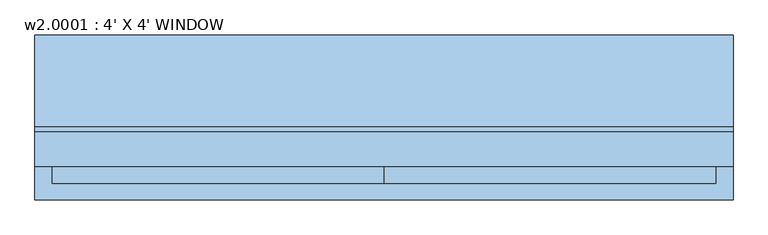
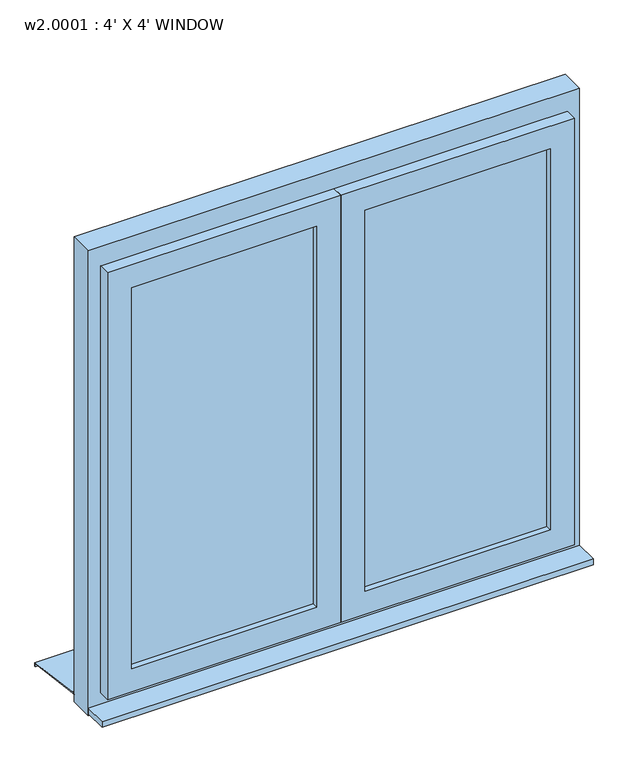
"""IFC4 building model written with IfcOpenShell, lengths in millimetres: window geometry, w2.0001 : 4' X 4' WINDOW."""

from ifc_helpers import new_model, si_unit, frame, origin, place, context, project, spatial, polyline, outline, extrude, faceted_brep, source, transform, mapped, element, save


def w2_0001_4_x_4_window_9dec5fc7(model_context):
    return source(origin(), model_context, "Body", "SolidModel", [
        extrude(outline(polyline([(-15.6778457, 1020.0), (144.3, 1000.0), (144.3, 990.0), (142.3, 990.0), (142.3, 998.3604634), (-15.8759277, 1018.0), (-25.7, 1018.0), (-25.7, 1020.0), (-15.6778457, 1020.0)])), frame((-609.6, 0.0, 0.0), z_axis=(1.0, 0.0, 0.0), x_axis=(0.0, 1.0, 0.0)), (0.0, 0.0, 1.0), 1219.2),
        extrude(outline(polyline([(-609.6, -144.3), (-609.6, -85.7), (609.6, -85.7), (609.6, -144.3), (-609.6, -144.3)])), frame((0.0, 0.0, 1005.0), z_axis=(0.0, 0.0, 1.0), x_axis=(1.0, 0.0, 0.0)), (0.0, 0.0, 1.0), 15.0),
        extrude(outline(polyline([(60.0, -70.7), (519.6, -70.7), (519.6, -100.7), (60.0, -100.7), (60.0, -70.7)])), frame((0.0, 0.0, 1110.0), z_axis=(0.0, 0.0, 1.0), x_axis=(1.0, 0.0, 0.0)), (0.0, 0.0, 1.0), 999.2),
        extrude(outline(polyline([(-519.6, -70.7), (-60.0, -70.7), (-60.0, -100.7), (-519.6, -100.7), (-519.6, -70.7)])), frame((0.0, 0.0, 1110.0), z_axis=(0.0, 0.0, 1.0), x_axis=(1.0, 0.0, 0.0)), (0.0, 0.0, 1.0), 999.2),
        extrude(outline(polyline([(2219.2, -609.6), (1000.0, -609.6), (1000.0, 609.6), (2219.2, 609.6), (2219.2, -609.6)]), holes=[polyline([(2139.2, -549.6), (2139.2, 549.6), (1080.0, 549.6), (1080.0, -549.6), (2139.2, -549.6)])]), frame((0.0, -85.7, 0.0), z_axis=(0.0, 1.0, 0.0), x_axis=(0.0, 0.0, 1.0)), (0.0, 0.0, 1.0), 60.0),
        extrude(outline(polyline([(30.0, -85.7), (-30.0, -85.7), (-30.0, -25.7), (30.0, -25.7), (30.0, -85.7)])), frame((0.0, 0.0, 1080.0), z_axis=(0.0, 0.0, 1.0), x_axis=(1.0, 0.0, 0.0)), (0.0, 0.0, 1.0), 1059.2),
        faceted_brep([(30.0, -85.7, 1080.0), (30.0, -55.7, 1080.0), (549.6, -55.7, 1080.0), (549.6, -85.7, 1080.0), (549.6, -55.7, 2139.2), (549.6, -85.7, 2139.2), (30.0, -55.7, 2139.2), (519.6, -55.7, 2109.2), (60.0, -55.7, 2109.2), (60.0, -55.7, 1110.0), (519.6, -55.7, 1110.0), (579.6, -85.7, 1050.0), (0.0, -85.7, 1050.0), (0.0, -85.7, 2169.2), (579.6, -85.7, 2169.2), (30.0, -85.7, 2139.2), (0.0, -115.7, 1050.0), (579.6, -115.7, 1050.0), (579.6, -115.7, 2169.2), (0.0, -115.7, 2169.2), (519.6, -115.7, 1110.0), (60.0, -115.7, 1110.0), (60.0, -115.7, 2109.2), (519.6, -115.7, 2109.2)], [[[0, 1, 2, 3]], [[3, 2, 4, 5]], [[2, 1, 6, 4], [7, 8, 9, 10]], [[11, 12, 13, 14], [5, 15, 0, 3]], [[16, 12, 11, 17]], [[17, 11, 14, 18]], [[18, 19, 16, 17], [20, 21, 22, 23]], [[9, 21, 20, 10]], [[10, 20, 23, 7]], [[15, 6, 1, 0]], [[19, 13, 12, 16]], [[8, 22, 21, 9]], [[5, 4, 6, 15]], [[18, 14, 13, 19]], [[7, 23, 22, 8]]]),
        faceted_brep([(-549.6, -85.7, 1080.0), (-549.6, -55.7, 1080.0), (-30.0, -55.7, 1080.0), (-30.0, -85.7, 1080.0), (-30.0, -55.7, 2139.2), (-30.0, -85.7, 2139.2), (-549.6, -55.7, 2139.2), (-60.0, -55.7, 2109.2), (-519.6, -55.7, 2109.2), (-519.6, -55.7, 1110.0), (-60.0, -55.7, 1110.0), (0.0, -85.7, 1050.0), (-579.6, -85.7, 1050.0), (-579.6, -85.7, 2169.2), (0.0, -85.7, 2169.2), (-549.6, -85.7, 2139.2), (-579.6, -115.7, 1050.0), (0.0, -115.7, 1050.0), (0.0, -115.7, 2169.2), (-579.6, -115.7, 2169.2), (-60.0, -115.7, 1110.0), (-519.6, -115.7, 1110.0), (-519.6, -115.7, 2109.2), (-60.0, -115.7, 2109.2)], [[[0, 1, 2, 3]], [[3, 2, 4, 5]], [[2, 1, 6, 4], [7, 8, 9, 10]], [[11, 12, 13, 14], [5, 15, 0, 3]], [[16, 12, 11, 17]], [[17, 11, 14, 18]], [[18, 19, 16, 17], [20, 21, 22, 23]], [[9, 21, 20, 10]], [[10, 20, 23, 7]], [[15, 6, 1, 0]], [[19, 13, 12, 16]], [[8, 22, 21, 9]], [[5, 4, 6, 15]], [[18, 14, 13, 19]], [[7, 23, 22, 8]]]),
    ])


if __name__ == "__main__":
    model = new_model("IFC4")
    model_context = context("Model", 3, world=origin())
    ifc_project = project(units=[si_unit("LENGTHUNIT", "METRE", prefix="MILLI")], contexts=[model_context])
    site = spatial("IfcSite", under=ifc_project)
    building = spatial("IfcBuilding", under=site)
    placement = place(None, origin())
    w2_0001_4_x_4_window_shape = w2_0001_4_x_4_window_9dec5fc7(model_context)
    element("IfcWindow", 1, ObjectType="w2.0001 : 4' X 4' WINDOW", at=placement, inside=building, context=model_context, shape_type="MappedRepresentation", body=[
        mapped(w2_0001_4_x_4_window_shape, transform((0.0, 0.0, 0.0), x_axis=(1.0, 0.0, 0.0), y_axis=(0.0, 1.0, 0.0), z_axis=(0.0, 0.0, 1.0))),
    ])
    save(model, "model.ifc")

# Revit data of these elements
# Type "w2.0001 : 4' X 4' WINDOW"
#   Type Mark = "21"
#   Operation = "DoublePanelVertical"
#   Keynote = "16.05.01"
#   Analytic Construction = "<None>"
#   Rough Width = 4' - 0"
#   Rough Height = 4' - 0"
#   Rahmentiefe = 0' - 2.3622"
#   Rahmenhöhe unten = 0' - 3.14961"
#   Rahmehöhe oben = 0' - 3.14961"
#   Rahmenbreite = 0' - 2.3622"
#   Height = 4' - 0"
#   Flügeltiefe = 0' - 2.3622"
#   Flügelbreite = 0' - 2.3622"
#   Einbautiefe (von außen) [instance default] = 0' - 5.51181"
#   Width = 4' - 0"
#   Kippflügel [instance default] = yes
#   Drehflügel im Grundriß darstellen [instance default] = no
#   Drehflügel [instance default] = yes
#   Define Thermal Properties by = 1
#   Rahmen [instance default] = none
#   Glas [instance default] = none
#   Flügel [instance default] = none
#   Fensterbank aussen [instance default] = none
#   Fensterbank innen [instance default] = none
#   Wall Closure = (empty or 0)
# Element 1 (IfcWindow, "w2.0001 : 4' X 4' WINDOW")
#   Materials on its faces: "Fenster - Kunststoff", "Fenster - Kunststoff weiss", "Glass", "Fenster - Holz"
# Materials
#   "Fenster - Kunststoff": colour RGB 249 249 249, transparency 0
#   "Fenster - Kunststoff weiss": colour RGB 249 249 249, transparency 0
#   "Glass": class "Glass", colour RGB 0 128 192, transparency 0.75, Description = "Soda Lime Glass", Cost = 0
#   "Fenster - Holz": colour RGB 216 135 75, transparency 0
